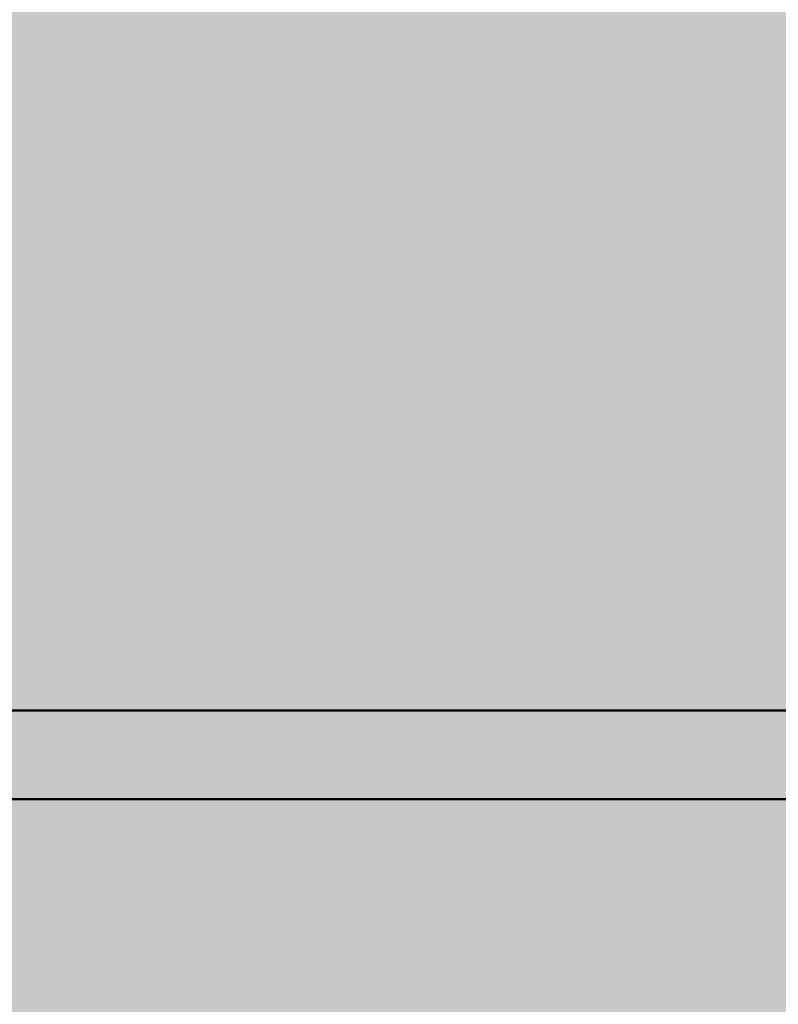
# Model space of a CAD drawing. Units: millimetres. Extents: x 0 to 2267, y 0 to 1823.
# Tile 134 of 256: x 1632 to 1675, y 1216 to 1271. Entities that reach past the tile are written whole.
import ezdxf

# ---------------------------------------------------------------- set-up
doc = ezdxf.new("R2010")
doc.units = ezdxf.units.MM
doc.header["$MEASUREMENT"] = 0
doc.layers.add('M-HATC', color=252, linetype='Continuous', lineweight=18)
doc.layers.add('M-OUTL', color=7, linetype='Continuous', lineweight=50)

msp = doc.modelspace()

# ---------------------------------------------------------------- hatches: boundary and pattern name
at = {"layer": 'M-HATC'}
h = msp.add_hatch(color=256, dxfattribs=at)
h.dxf.hatch_style = 1
h.paths.add_polyline_path([(2065.771, 1618.062, 0.236068), (2055.771, 1638.062), (1381.087, 1638.062, 0.236068), (1371.087, 1618.062), (1371.087, 1603.062), (2055.771, 1603.062), (2065.771, 1603.062)])
h.paths.add_polyline_path([(2062.772, 1550.296), (2062.772, 1560.296), (1374.086, 1560.296), (1374.086, 1550.296), (1374.086, 1540.296), (1384.086, 1540.296), (1389.086, 1540.296), (2062.772, 1540.296)])
h.paths.add_polyline_path([(1930.929, 1282.766), (1505.929, 1282.766), (1587.628, 1235.597, 0.131652), (1600.128, 1232.247), (1836.73, 1232.247, 0.131652), (1849.23, 1235.597)])
h.paths.add_polyline_path([(1930.929, 1117.417), (1905.929, 1117.417), (1505.929, 1117.417), (1505.929, 1077.417), (1930.929, 1077.417)])
h = msp.add_hatch(color=256, dxfattribs=at)
h.dxf.hatch_style = 1
h.paths.add_polyline_path([(2055.771, 1603.062), (1381.087, 1603.062), (1381.087, 1598.062), (2055.771, 1598.062)])
h.paths.add_polyline_path([(2055.771, 1598.062), (1381.087, 1598.062), (1381.087, 1593.062), (2055.771, 1593.062)])
h.paths.add_polyline_path([(2051.307, 1536.761), (1385.55, 1536.761), (1385.55, 1526.761), (1387.55, 1526.761), (1388.537, 1525.053), (1385.332, 1521.233), (1385.332, 1521.223), (2050.254, 1522.749), (2048.321, 1525.053), (2049.307, 1526.761), (2051.307, 1526.761)])
edge = h.paths.add_edge_path()
edge.add_arc((1847.535, 1379.149), 135, 222.60306, 222.89085, ccw=False)
edge.add_line((1748.166, 1287.766), (1683.092, 1287.766))
edge.add_arc((1583.724, 1379.149), 135, 317.10915, 317.39694, ccw=False)
edge.add_arc((1678.969, 1290.671), 5, 222.8909, 317.1091, ccw=False)
edge.add_arc((1774.213, 1379.149), 135, 222.60306, 222.89085, ccw=False)
edge.add_line((1674.845, 1287.766), (1609.771, 1287.766))
edge.add_arc((1510.403, 1379.149), 135, 317.10915, 317.39694, ccw=False)
edge.add_arc((1605.647, 1290.671), 5, 222.8909, 317.1091, ccw=False)
edge.add_arc((1700.892, 1379.149), 135, 222.60306, 222.89085, ccw=False)
edge.add_line((1601.524, 1287.766), (1536.45, 1287.766))
edge.add_arc((1437.081, 1379.149), 135, 317.10915, 317.39694, ccw=False)
edge.add_arc((1532.326, 1290.671), 5, 222.8909, 317.1091, ccw=False)
edge.add_arc((1627.571, 1379.149), 135, 222.60306, 222.89085, ccw=False)
edge.add_line((1528.203, 1287.766), (1505.929, 1287.766))
edge.add_spline(control_points=[(1505.929, 1287.766), (1504.262, 1287.766), (1504.262, 1282.766), (1505.929, 1282.766)], knot_values=[0, 0, 0, 0, 5, 5, 5, 5], degree=3, periodic=0)
edge.add_line((1505.929, 1282.766), (1930.929, 1282.766))
edge.add_spline(control_points=[(1930.929, 1282.766), (1932.596, 1282.766), (1932.596, 1287.766), (1930.929, 1287.766)], knot_values=[0, 0, 0, 0, 5, 5, 5, 5], degree=3, periodic=0)
edge.add_line((1930.929, 1287.766), (1903.056, 1287.766))
edge.add_arc((1803.688, 1379.149), 135, 317.10915, 317.39694, ccw=False)
edge.add_arc((1898.932, 1290.671), 5, 222.8909, 317.1091, ccw=False)
edge.add_arc((1994.177, 1379.149), 135, 222.60306, 222.89085, ccw=False)
edge.add_line((1894.809, 1287.766), (1829.735, 1287.766))
edge.add_arc((1730.366, 1379.149), 135, 317.10915, 317.39694, ccw=False)
edge.add_arc((1825.611, 1290.671), 5, 222.8909, 317.1091, ccw=False)
edge.add_arc((1920.856, 1379.149), 135, 222.60306, 222.89085, ccw=False)
edge.add_line((1821.487, 1287.766), (1756.413, 1287.766))
edge.add_arc((1657.045, 1379.149), 135, 317.10915, 317.39694, ccw=False)
edge.add_arc((1752.29, 1290.671), 5, 222.8909, 317.1091, ccw=False)
edge = h.paths.add_edge_path()
edge.add_spline(control_points=[(1843.429, 1227.247), (1845.096, 1227.247), (1845.096, 1232.247), (1843.429, 1232.247)], knot_values=[0, 0, 0, 0, 5, 5, 5, 5], degree=3, periodic=0)
edge.add_line((1843.429, 1232.247), (1593.429, 1232.247))
edge.add_spline(control_points=[(1593.429, 1232.247), (1591.762, 1232.247), (1591.762, 1227.247), (1593.429, 1227.247)], knot_values=[0, 0, 0, 0, 5, 5, 5, 5], degree=3, periodic=0)
edge.add_line((1593.429, 1227.247), (1843.429, 1227.247))
h.paths.add_polyline_path([(1905.929, 1127.417), (1530.929, 1127.417, 0.414214), (1520.929, 1117.417), (1530.929, 1117.417), (1915.929, 1117.417, 0.414214)])
edge = h.paths.add_edge_path()
edge.add_arc((1397.086, 1498.408), 12.73, 90.7821, 190.8787, ccw=False)
edge.add_line((1396.912, 1511.136), (1428.01, 1511.349))
edge.add_line((1428.01, 1511.349), (1433.01, 1511.349))
edge.add_line((1433.01, 1511.349), (1434.439, 1511.349))
edge.add_arc((1419.474, 1498.08), 20, 41.561, 74.0821)
edge.add_line((1424.959, 1517.314), (1399.935, 1517.256))
edge.add_spline(control_points=[(1399.931, 1517.256), (1399.884, 1517.213), (1399.833, 1517.169), (1399.777, 1517.124)], knot_values=[11.567499, 11.567499, 11.567499, 11.567499, 11.814249, 11.814249, 11.814249, 11.814249], degree=3, periodic=0)
edge.add_spline(control_points=[(1399.633, 1517.01), (1399.583, 1516.972), (1399.531, 1516.934), (1399.476, 1516.895)], knot_values=[11.167718, 11.167718, 11.167718, 11.167718, 11.365188, 11.365188, 11.365188, 11.365188], degree=3, periodic=0)
edge.add_spline(control_points=[(1399.34, 1516.8), (1399.151, 1516.672), (1398.938, 1516.538), (1398.704, 1516.399)], knot_values=[10.376405, 10.376405, 10.376405, 10.376405, 11.00994, 11.00994, 11.00994, 11.00994], degree=3, periodic=0)
edge.add_spline(control_points=[(1398.657, 1516.372), (1398.579, 1516.326), (1398.498, 1516.28), (1398.415, 1516.233)], knot_values=[10.125175, 10.125175, 10.125175, 10.125175, 10.334406, 10.334406, 10.334406, 10.334406], degree=3, periodic=0)
edge.add_spline(control_points=[(1398.264, 1516.149), (1398.196, 1516.111), (1398.126, 1516.073), (1398.055, 1516.035)], knot_values=[9.832246, 9.832246, 9.832246, 9.832246, 9.999658, 9.999658, 9.999658, 9.999658], degree=3, periodic=0)
edge.add_spline(control_points=[(1397.999, 1516.005), (1397.731, 1515.862), (1397.446, 1515.717), (1397.147, 1515.571)], knot_values=[9.161808, 9.161808, 9.161808, 9.161808, 9.787769, 9.787769, 9.787769, 9.787769], degree=3, periodic=0)
edge.add_spline(control_points=[(1397.147, 1515.571), (1396.842, 1515.423), (1396.522, 1515.274), (1396.191, 1515.126)], knot_values=[8.524455, 8.524455, 8.524455, 8.524455, 9.161808, 9.161808, 9.161808, 9.161808], degree=3, periodic=0)
edge.add_spline(control_points=[(1396.078, 1515.076), (1395.985, 1515.035), (1395.892, 1514.994), (1395.798, 1514.953)], knot_values=[8.275193, 8.275193, 8.275193, 8.275193, 8.451726, 8.451726, 8.451726, 8.451726], degree=3, periodic=0)
edge.add_spline(control_points=[(1395.602, 1514.869), (1395.5, 1514.826), (1395.397, 1514.782), (1395.293, 1514.739)], knot_values=[7.962917, 7.962917, 7.962917, 7.962917, 8.152764, 8.152764, 8.152764, 8.152764], degree=3, periodic=0)
edge.add_spline(control_points=[(1395.212, 1514.706), (1394.828, 1514.547), (1394.435, 1514.393), (1394.036, 1514.244)], knot_values=[7.21254, 7.21254, 7.21254, 7.21254, 7.913148, 7.913148, 7.913148, 7.913148], degree=3, periodic=0)
edge.add_spline(control_points=[(1394.036, 1514.244), (1393.708, 1514.121), (1393.375, 1514.003), (1393.043, 1513.889)], knot_values=[6.633733, 6.633733, 6.633733, 6.633733, 7.21254, 7.21254, 7.21254, 7.21254], degree=3, periodic=0)
edge.add_spline(control_points=[(1392.821, 1513.815), (1392.72, 1513.781), (1392.618, 1513.748), (1392.517, 1513.715)], knot_values=[6.328796, 6.328796, 6.328796, 6.328796, 6.505493, 6.505493, 6.505493, 6.505493], degree=3, periodic=0)
edge.add_spline(control_points=[(1392.517, 1513.715), (1392.319, 1513.652), (1392.121, 1513.59), (1391.924, 1513.531)], knot_values=[5.984605, 5.984605, 5.984605, 5.984605, 6.328796, 6.328796, 6.328796, 6.328796], degree=3, periodic=0)
edge.add_spline(control_points=[(1391.792, 1513.491), (1391.312, 1513.35), (1390.838, 1513.224), (1390.378, 1513.117)], knot_values=[5.066697, 5.066697, 5.066697, 5.066697, 5.907055, 5.907055, 5.907055, 5.907055], degree=3, periodic=0)
edge.add_spline(control_points=[(1390.378, 1513.117), (1390.18, 1513.071), (1389.984, 1513.028), (1389.791, 1512.99)], knot_values=[4.70367, 4.70367, 4.70367, 4.70367, 5.066695, 5.066695, 5.066695, 5.066695], degree=3, periodic=0)
edge.add_spline(control_points=[(1389.422, 1512.92), (1389.246, 1512.889), (1389.073, 1512.862), (1388.904, 1512.838)], knot_values=[4.130571, 4.130571, 4.130571, 4.130571, 4.469816, 4.469816, 4.469816, 4.469816], degree=3, periodic=0)
edge.add_spline(control_points=[(1388.904, 1512.838), (1388.591, 1512.795), (1388.291, 1512.764), (1388.007, 1512.749)], knot_values=[3.504031, 3.504031, 3.504031, 3.504031, 4.130571, 4.130571, 4.130571, 4.130571], degree=3, periodic=0)
edge.add_spline(control_points=[(1387.936, 1512.746), (1387.854, 1512.742), (1387.773, 1512.74), (1387.694, 1512.739)], knot_values=[3.268866, 3.268866, 3.268866, 3.268866, 3.451164, 3.451164, 3.451164, 3.451164], degree=3, periodic=0)
edge.add_spline(control_points=[(1387.335, 1512.744), (1387.208, 1512.75), (1387.085, 1512.76), (1386.967, 1512.774)], knot_values=[2.670686, 2.670686, 2.670686, 2.670686, 2.984, 2.984, 2.984, 2.984], degree=3, periodic=0)
edge.add_spline(control_points=[(1386.833, 1512.792), (1386.821, 1512.794), (1386.809, 1512.796), (1386.797, 1512.798)], knot_values=[2.516981, 2.516981, 2.516981, 2.516981, 2.549528, 2.549528, 2.549528, 2.549528], degree=3, periodic=0)
edge.add_spline(control_points=[(1386.453, 1512.873), (1386.426, 1512.881), (1386.399, 1512.889), (1386.373, 1512.897)], knot_values=[2.095869, 2.095869, 2.095869, 2.095869, 2.17941, 2.17941, 2.17941, 2.17941], degree=3, periodic=0)
edge.add_spline(control_points=[(1386.069, 1513.019), (1386.063, 1513.022), (1386.058, 1513.025), (1386.052, 1513.028)], knot_values=[1.72453, 1.72453, 1.72453, 1.72453, 1.745933, 1.745933, 1.745933, 1.745933], degree=3, periodic=0)
edge.add_arc((1399.474, 1498.08), 20, 131.8243, 180)
edge.add_arc((1630.334, 1505.548), 250.971, 181.70518, 236.42798)
edge.add_arc((1605.34, 1483.304), 218.782, 238.66083, 243.34961)
edge.add_arc((1647.091, 1510.359), 262.899, 183.12984, 237.85344, ccw=False)
h.paths.add_polyline_path([(1406.537, 1391.964, 0.149382), (1491.551, 1296.442, -0.129517)], flags=17)
edge = h.paths.add_edge_path()
edge.add_arc((2037.384, 1498.08), 20, 0, 48.2659)
edge.add_spline(control_points=[(2050.697, 1513.005), (2050.651, 1512.985), (2050.603, 1512.966), (2050.554, 1512.948)], knot_values=[1.835652, 1.835652, 1.835652, 1.835652, 2.000781, 2.000781, 2.000781, 2.000781], degree=3, periodic=0)
edge.add_spline(control_points=[(2050.462, 1512.917), (2050.479, 1512.922), (2050.496, 1512.928), (2050.513, 1512.934)], knot_values=[2.045477, 2.045477, 2.045477, 2.045477, 2.101389, 2.101389, 2.101389, 2.101389], degree=3, periodic=0)
edge.add_spline(control_points=[(2050.129, 1512.834), (2050.198, 1512.847), (2050.266, 1512.862), (2050.331, 1512.879)], knot_values=[2.237629, 2.237629, 2.237629, 2.237629, 2.435841, 2.435841, 2.435841, 2.435841], degree=3, periodic=0)
edge.add_spline(control_points=[(2050.095, 1512.828), (2050.106, 1512.83), (2050.118, 1512.832), (2050.129, 1512.834)], knot_values=[2.435841, 2.435841, 2.435841, 2.435841, 2.468321, 2.468321, 2.468321, 2.468321], degree=3, periodic=0)
edge.add_spline(control_points=[(2049.784, 1512.785), (2049.855, 1512.792), (2049.924, 1512.801), (2049.992, 1512.811)], knot_values=[2.563852, 2.563852, 2.563852, 2.563852, 2.748541, 2.748541, 2.748541, 2.748541], degree=3, periodic=0)
edge.add_spline(control_points=[(2049.405, 1512.762), (2049.536, 1512.765), (2049.663, 1512.773), (2049.784, 1512.785)], knot_values=[2.748541, 2.748541, 2.748541, 2.748541, 3.064882, 3.064882, 3.064882, 3.064882], degree=3, periodic=0)
edge.add_spline(control_points=[(2049.17, 1512.76), (2049.234, 1512.759), (2049.297, 1512.759), (2049.358, 1512.761)], knot_values=[3.102309, 3.102309, 3.102309, 3.102309, 3.2503, 3.2503, 3.2503, 3.2503], degree=3, periodic=0)
edge.add_spline(control_points=[(2048.857, 1512.769), (2048.964, 1512.764), (2049.068, 1512.761), (2049.17, 1512.76)], knot_values=[3.2503, 3.2503, 3.2503, 3.2503, 3.486069, 3.486069, 3.486069, 3.486069], degree=3, periodic=0)
edge.add_spline(control_points=[(2048.692, 1512.779), (2048.373, 1512.801), (2048.035, 1512.841), (2047.682, 1512.897)], knot_values=[3.606429, 3.606429, 3.606429, 3.606429, 4.2989, 4.2989, 4.2989, 4.2989], degree=3, periodic=0)
edge.add_spline(control_points=[(2047.682, 1512.897), (2047.546, 1512.919), (2047.408, 1512.942), (2047.268, 1512.969)], knot_values=[4.2989, 4.2989, 4.2989, 4.2989, 4.565769, 4.565769, 4.565769, 4.565769], degree=3, periodic=0)
edge.add_spline(control_points=[(2047.268, 1512.969), (2047.145, 1512.991), (2047.021, 1513.016), (2046.895, 1513.042)], knot_values=[4.565769, 4.565769, 4.565769, 4.565769, 4.799971, 4.799971, 4.799971, 4.799971], degree=3, periodic=0)
edge.add_spline(control_points=[(2046.895, 1513.042), (2046.529, 1513.119), (2046.151, 1513.209), (2045.768, 1513.311)], knot_values=[4.799971, 4.799971, 4.799971, 4.799971, 5.483718, 5.483718, 5.483718, 5.483718], degree=3, periodic=0)
edge.add_spline(control_points=[(2045.768, 1513.311), (2045.372, 1513.415), (2044.97, 1513.532), (2044.566, 1513.659)], knot_values=[5.483718, 5.483718, 5.483718, 5.483718, 6.187866, 6.187866, 6.187866, 6.187866], degree=3, periodic=0)
edge.add_spline(control_points=[(2044.566, 1513.659), (2044.415, 1513.706), (2044.263, 1513.755), (2044.112, 1513.805)], knot_values=[6.187866, 6.187866, 6.187866, 6.187866, 6.451551, 6.451551, 6.451551, 6.451551], degree=3, periodic=0)
edge.add_spline(control_points=[(2044.112, 1513.805), (2043.997, 1513.843), (2043.882, 1513.881), (2043.767, 1513.92)], knot_values=[6.451551, 6.451551, 6.451551, 6.451551, 6.651434, 6.651434, 6.651434, 6.651434], degree=3, periodic=0)
edge.add_spline(control_points=[(2043.767, 1513.92), (2043.372, 1514.055), (2042.977, 1514.198), (2042.589, 1514.346)], knot_values=[6.651434, 6.651434, 6.651434, 6.651434, 7.338879, 7.338879, 7.338879, 7.338879], degree=3, periodic=0)
edge.add_spline(control_points=[(2042.589, 1514.346), (2042.164, 1514.507), (2041.746, 1514.675), (2041.341, 1514.846)], knot_values=[7.338879, 7.338879, 7.338879, 7.338879, 8.089209, 8.089209, 8.089209, 8.089209], degree=3, periodic=0)
edge.add_spline(control_points=[(2041.341, 1514.846), (2041.103, 1514.946), (2040.869, 1515.048), (2040.64, 1515.15)], knot_values=[8.089209, 8.089209, 8.089209, 8.089209, 8.529587, 8.529587, 8.529587, 8.529587], degree=3, periodic=0)
edge.add_spline(control_points=[(2040.51, 1515.209), (2040.082, 1515.402), (2039.675, 1515.597), (2039.295, 1515.789)], knot_values=[8.613818, 8.613818, 8.613818, 8.613818, 9.44571, 9.44571, 9.44571, 9.44571], degree=3, periodic=0)
edge.add_spline(control_points=[(2039.295, 1515.789), (2039.062, 1515.907), (2038.839, 1516.025), (2038.629, 1516.14)], knot_values=[9.44571, 9.44571, 9.44571, 9.44571, 9.956404, 9.956404, 9.956404, 9.956404], degree=3, periodic=0)
edge.add_spline(control_points=[(2038.629, 1516.14), (2038.519, 1516.2), (2038.412, 1516.26), (2038.309, 1516.319)], knot_values=[9.956404, 9.956404, 9.956404, 9.956404, 10.223542, 10.223542, 10.223542, 10.223542], degree=3, periodic=0)
edge.add_spline(control_points=[(2038.309, 1516.319), (2038.214, 1516.374), (2038.122, 1516.428), (2038.033, 1516.481)], knot_values=[10.223542, 10.223542, 10.223542, 10.223542, 10.47051, 10.47051, 10.47051, 10.47051], degree=3, periodic=0)
edge.add_spline(control_points=[(2038.033, 1516.481), (2037.786, 1516.63), (2037.564, 1516.773), (2037.372, 1516.909)], knot_values=[10.47051, 10.47051, 10.47051, 10.47051, 11.15767, 11.15767, 11.15767, 11.15767], degree=3, periodic=0)
edge.add_spline(control_points=[(2037.372, 1516.909), (2037.279, 1516.975), (2037.193, 1517.04), (2037.114, 1517.102)], knot_values=[11.15767, 11.15767, 11.15767, 11.15767, 11.49227, 11.49227, 11.49227, 11.49227], degree=3, periodic=0)
edge.add_spline(control_points=[(2036.856, 1517.326), (2036.915, 1517.269), (2036.981, 1517.21), (2037.056, 1517.149)], knot_values=[11.577341, 11.577341, 11.577341, 11.577341, 11.91035, 11.91035, 11.91035, 11.91035], degree=3, periodic=0)
edge.add_spline(control_points=[(2036.807, 1517.375), (2036.823, 1517.359), (2036.839, 1517.342), (2036.856, 1517.326)], knot_values=[11.91035, 11.91035, 11.91035, 11.91035, 12.007402, 12.007402, 12.007402, 12.007402], degree=3, periodic=0)
edge.add_spline(control_points=[(2036.702, 1517.494), (2036.71, 1517.483), (2036.72, 1517.472), (2036.729, 1517.461)], knot_values=[12.184155, 12.184155, 12.184155, 12.184155, 12.255409, 12.255409, 12.255409, 12.255409], degree=3, periodic=0)
edge.add_spline(control_points=[(2036.616, 1517.621), (2036.62, 1517.613), (2036.624, 1517.606), (2036.629, 1517.598)], knot_values=[12.487913, 12.487913, 12.487913, 12.487913, 12.541035, 12.541035, 12.541035, 12.541035], degree=3, periodic=0)
edge.add_spline(control_points=[(2036.563, 1517.786), (2036.564, 1517.779), (2036.564, 1517.773), (2036.565, 1517.766)], knot_values=[12.911761, 12.911761, 12.911761, 12.911761, 12.968286, 12.968286, 12.968286, 12.968286], degree=3, periodic=0)
edge.add_spline(control_points=[(2036.617, 1517.93), (2036.612, 1517.926), (2036.609, 1517.921), (2036.605, 1517.916)], knot_values=[13.382527, 13.382527, 13.382527, 13.382527, 13.433791, 13.433791, 13.433791, 13.433791], degree=3, periodic=0)
edge.add_spline(control_points=[(2036.749, 1518.017), (2036.736, 1518.012), (2036.724, 1518.006), (2036.712, 1518)], knot_values=[13.726299, 13.726299, 13.726299, 13.726299, 13.809928, 13.809928, 13.809928, 13.809928], degree=3, periodic=0)
edge.add_spline(control_points=[(2036.86, 1518.053), (2036.839, 1518.047), (2036.818, 1518.042), (2036.799, 1518.035)], knot_values=[13.910887, 13.910887, 13.910887, 13.910887, 14.02153, 14.02153, 14.02153, 14.02153], degree=3, periodic=0)
edge.add_line((2036.964, 1518.08), (2032.384, 1518.08))
edge.add_line((2032.384, 1518.08), (2027.384, 1518.08))
edge.add_line((2027.384, 1518.08), (2022.384, 1518.08))
edge.add_line((2022.384, 1518.08), (2017.384, 1518.08))
edge.add_arc((2017.384, 1498.08), 20, 90, 138.439)
edge.add_line((2002.419, 1511.349), (2003.848, 1511.349))
edge.add_line((2003.848, 1511.349), (2008.848, 1511.349))
edge.add_line((2008.848, 1511.349), (2039.772, 1511.138))
edge.add_arc((2039.772, 1498.408), 12.73, -10.8787, 90, ccw=False)
edge.add_arc((1789.767, 1510.359), 262.899, 302.14656, 356.87016, ccw=False)
edge.add_arc((1831.518, 1483.304), 218.782, 296.65039, 301.33917)
edge.add_arc((1806.524, 1505.548), 250.971, 303.57202, 358.29482)
h.paths.add_polyline_path([(2030.321, 1391.964, -0.129517), (1945.307, 1296.442, 0.149382)], flags=17)
edge = h.paths.add_edge_path()
edge.add_spline(control_points=[(2037.246, 1518.082), (2037.29, 1518.081), (2037.336, 1518.08), (2037.384, 1518.08)], knot_values=[0.000012, 0.000012, 0.000012, 0.000012, 0.144754, 0.144754, 0.144754, 0.144754], degree=3, periodic=0)
edge.add_line((2037.336, 1518.08), (2037.01, 1518.08))
edge.add_spline(control_points=[(2037.01, 1518.08), (2036.982, 1518.077), (2036.956, 1518.073), (2036.931, 1518.068)], knot_values=[14.13465, 14.13465, 14.13465, 14.13465, 14.247197, 14.247197, 14.247197, 14.247197], degree=3, periodic=0)
edge.add_spline(control_points=[(2036.931, 1518.068), (2036.928, 1518.067), (2036.924, 1518.067), (2036.921, 1518.066)], knot_values=[14.118315, 14.118315, 14.118315, 14.118315, 14.13465, 14.13465, 14.13465, 14.13465], degree=3, periodic=0)
edge.add_spline(control_points=[(2036.921, 1518.066), (2036.912, 1518.064), (2036.903, 1518.063), (2036.895, 1518.061)], knot_values=[14.078086, 14.078086, 14.078086, 14.078086, 14.118315, 14.118315, 14.118315, 14.118315], degree=3, periodic=0)
edge.add_spline(control_points=[(2036.895, 1518.061), (2036.883, 1518.058), (2036.872, 1518.056), (2036.86, 1518.053)], knot_values=[14.02153, 14.02153, 14.02153, 14.02153, 14.078086, 14.078086, 14.078086, 14.078086], degree=3, periodic=0)
edge.add_spline(control_points=[(2036.86, 1518.053), (2036.839, 1518.047), (2036.818, 1518.042), (2036.799, 1518.035)], knot_values=[13.910887, 13.910887, 13.910887, 13.910887, 14.02153, 14.02153, 14.02153, 14.02153], degree=3, periodic=0)
edge.add_spline(control_points=[(2036.799, 1518.035), (2036.798, 1518.035), (2036.797, 1518.035), (2036.797, 1518.035)], knot_values=[13.906906, 13.906906, 13.906906, 13.906906, 13.910887, 13.910887, 13.910887, 13.910887], degree=3, periodic=0)
edge.add_spline(control_points=[(2036.797, 1518.035), (2036.788, 1518.032), (2036.78, 1518.029), (2036.772, 1518.026)], knot_values=[13.857826, 13.857826, 13.857826, 13.857826, 13.906906, 13.906906, 13.906906, 13.906906], degree=3, periodic=0)
edge.add_spline(control_points=[(2036.772, 1518.026), (2036.764, 1518.023), (2036.756, 1518.02), (2036.749, 1518.017)], knot_values=[13.809928, 13.809928, 13.809928, 13.809928, 13.857826, 13.857826, 13.857826, 13.857826], degree=3, periodic=0)
edge.add_spline(control_points=[(2036.749, 1518.017), (2036.736, 1518.012), (2036.724, 1518.006), (2036.712, 1518)], knot_values=[13.726299, 13.726299, 13.726299, 13.726299, 13.809928, 13.809928, 13.809928, 13.809928], degree=3, periodic=0)
edge.add_spline(control_points=[(2036.712, 1518), (2036.712, 1518), (2036.712, 1518), (2036.711, 1518)], knot_values=[13.723993, 13.723993, 13.723993, 13.723993, 13.726299, 13.726299, 13.726299, 13.726299], degree=3, periodic=0)
edge.add_spline(control_points=[(2036.711, 1518), (2036.706, 1517.997), (2036.701, 1517.994), (2036.696, 1517.992)], knot_values=[13.686536, 13.686536, 13.686536, 13.686536, 13.723993, 13.723993, 13.723993, 13.723993], degree=3, periodic=0)
edge.add_spline(control_points=[(2036.696, 1517.992), (2036.692, 1517.989), (2036.687, 1517.987), (2036.683, 1517.984)], knot_values=[13.651251, 13.651251, 13.651251, 13.651251, 13.686536, 13.686536, 13.686536, 13.686536], degree=3, periodic=0)
edge.add_spline(control_points=[(2036.683, 1517.984), (2036.676, 1517.98), (2036.67, 1517.976), (2036.664, 1517.971)], knot_values=[13.596804, 13.596804, 13.596804, 13.596804, 13.651251, 13.651251, 13.651251, 13.651251], degree=3, periodic=0)
edge.add_spline(control_points=[(2036.664, 1517.971), (2036.664, 1517.971), (2036.663, 1517.971), (2036.663, 1517.971)], knot_values=[13.593956, 13.593956, 13.593956, 13.593956, 13.596804, 13.596804, 13.596804, 13.596804], degree=3, periodic=0)
edge.add_spline(control_points=[(2036.663, 1517.971), (2036.66, 1517.969), (2036.658, 1517.967), (2036.655, 1517.965)], knot_values=[13.570322, 13.570322, 13.570322, 13.570322, 13.593956, 13.593956, 13.593956, 13.593956], degree=3, periodic=0)
edge.add_spline(control_points=[(2036.655, 1517.965), (2036.653, 1517.963), (2036.65, 1517.961), (2036.647, 1517.959)], knot_values=[13.545477, 13.545477, 13.545477, 13.545477, 13.570322, 13.570322, 13.570322, 13.570322], degree=3, periodic=0)
edge.add_spline(control_points=[(2036.647, 1517.959), (2036.647, 1517.959), (2036.647, 1517.959), (2036.647, 1517.959)], knot_values=[13.543931, 13.543931, 13.543931, 13.543931, 13.545477, 13.545477, 13.545477, 13.545477], degree=3, periodic=0)
edge.add_spline(control_points=[(2036.647, 1517.959), (2036.641, 1517.954), (2036.636, 1517.949), (2036.631, 1517.945)], knot_values=[13.488237, 13.488237, 13.488237, 13.488237, 13.543931, 13.543931, 13.543931, 13.543931], degree=3, periodic=0)
edge.add_spline(control_points=[(2036.631, 1517.945), (2036.628, 1517.942), (2036.626, 1517.94), (2036.623, 1517.937)], knot_values=[13.460307, 13.460307, 13.460307, 13.460307, 13.488237, 13.488237, 13.488237, 13.488237], degree=3, periodic=0)
edge.add_spline(control_points=[(2036.623, 1517.937), (2036.622, 1517.936), (2036.62, 1517.934), (2036.618, 1517.932)], knot_values=[13.439712, 13.439712, 13.439712, 13.439712, 13.460307, 13.460307, 13.460307, 13.460307], degree=3, periodic=0)
edge.add_spline(control_points=[(2036.618, 1517.932), (2036.618, 1517.931), (2036.617, 1517.931), (2036.617, 1517.93)], knot_values=[13.433791, 13.433791, 13.433791, 13.433791, 13.439712, 13.439712, 13.439712, 13.439712], degree=3, periodic=0)
edge.add_spline(control_points=[(2036.617, 1517.93), (2036.612, 1517.926), (2036.609, 1517.921), (2036.605, 1517.916)], knot_values=[13.382527, 13.382527, 13.382527, 13.382527, 13.433791, 13.433791, 13.433791, 13.433791], degree=3, periodic=0)
edge.add_spline(control_points=[(2036.605, 1517.916), (2036.603, 1517.913), (2036.6, 1517.91), (2036.598, 1517.907)], knot_values=[13.350017, 13.350017, 13.350017, 13.350017, 13.382527, 13.382527, 13.382527, 13.382527], degree=3, periodic=0)
edge.add_spline(control_points=[(2036.598, 1517.907), (2036.597, 1517.906), (2036.596, 1517.904), (2036.595, 1517.903)], knot_values=[13.333922, 13.333922, 13.333922, 13.333922, 13.350017, 13.350017, 13.350017, 13.350017], degree=3, periodic=0)
edge.add_spline(control_points=[(2036.595, 1517.903), (2036.595, 1517.902), (2036.594, 1517.901), (2036.593, 1517.9)], knot_values=[13.323828, 13.323828, 13.323828, 13.323828, 13.333922, 13.333922, 13.333922, 13.333922], degree=3, periodic=0)
edge.add_spline(control_points=[(2036.593, 1517.9), (2036.59, 1517.895), (2036.588, 1517.891), (2036.585, 1517.886)], knot_values=[13.277545, 13.277545, 13.277545, 13.277545, 13.323828, 13.323828, 13.323828, 13.323828], degree=3, periodic=0)
edge.add_spline(control_points=[(2036.585, 1517.886), (2036.584, 1517.883), (2036.582, 1517.879), (2036.58, 1517.875)], knot_values=[13.240119, 13.240119, 13.240119, 13.240119, 13.277545, 13.277545, 13.277545, 13.277545], degree=3, periodic=0)
edge.add_spline(control_points=[(2036.58, 1517.875), (2036.58, 1517.874), (2036.579, 1517.873), (2036.578, 1517.872)], knot_values=[13.228211, 13.228211, 13.228211, 13.228211, 13.240119, 13.240119, 13.240119, 13.240119], degree=3, periodic=0)
edge.add_spline(control_points=[(2036.578, 1517.872), (2036.578, 1517.87), (2036.577, 1517.869), (2036.577, 1517.868)], knot_values=[13.215717, 13.215717, 13.215717, 13.215717, 13.228211, 13.228211, 13.228211, 13.228211], degree=3, periodic=0)
edge.add_spline(control_points=[(2036.577, 1517.868), (2036.575, 1517.864), (2036.574, 1517.86), (2036.573, 1517.857)], knot_values=[13.179847, 13.179847, 13.179847, 13.179847, 13.215717, 13.215717, 13.215717, 13.215717], degree=3, periodic=0)
edge.add_spline(control_points=[(2036.573, 1517.857), (2036.571, 1517.851), (2036.57, 1517.846), (2036.569, 1517.841)], knot_values=[13.132017, 13.132017, 13.132017, 13.132017, 13.179847, 13.179847, 13.179847, 13.179847], degree=3, periodic=0)
edge.add_spline(control_points=[(2036.569, 1517.841), (2036.568, 1517.84), (2036.568, 1517.839), (2036.568, 1517.838)], knot_values=[13.122482, 13.122482, 13.122482, 13.122482, 13.132017, 13.132017, 13.132017, 13.132017], degree=3, periodic=0)
edge.add_spline(control_points=[(2036.568, 1517.838), (2036.568, 1517.836), (2036.567, 1517.835), (2036.567, 1517.833)], knot_values=[13.105592, 13.105592, 13.105592, 13.105592, 13.122482, 13.122482, 13.122482, 13.122482], degree=3, periodic=0)
edge.add_spline(control_points=[(2036.567, 1517.833), (2036.566, 1517.829), (2036.566, 1517.826), (2036.565, 1517.822)], knot_values=[13.074063, 13.074063, 13.074063, 13.074063, 13.105592, 13.105592, 13.105592, 13.105592], degree=3, periodic=0)
edge.add_spline(control_points=[(2036.565, 1517.822), (2036.565, 1517.822), (2036.565, 1517.822), (2036.565, 1517.822)], knot_values=[13.074043, 13.074043, 13.074043, 13.074043, 13.074063, 13.074063, 13.074063, 13.074063], degree=3, periodic=0)
edge.add_spline(control_points=[(2036.565, 1517.822), (2036.564, 1517.816), (2036.564, 1517.811), (2036.564, 1517.805)], knot_values=[13.021884, 13.021884, 13.021884, 13.021884, 13.074043, 13.074043, 13.074043, 13.074043], degree=3, periodic=0)
edge.add_spline(control_points=[(2036.564, 1517.805), (2036.564, 1517.804), (2036.564, 1517.803), (2036.564, 1517.803)], knot_values=[13.01674, 13.01674, 13.01674, 13.01674, 13.021884, 13.021884, 13.021884, 13.021884], degree=3, periodic=0)
edge.add_spline(control_points=[(2036.564, 1517.803), (2036.563, 1517.801), (2036.563, 1517.798), (2036.563, 1517.796)], knot_values=[12.996438, 12.996438, 12.996438, 12.996438, 13.01674, 13.01674, 13.01674, 13.01674], degree=3, periodic=0)
edge.add_spline(control_points=[(2036.563, 1517.796), (2036.563, 1517.793), (2036.563, 1517.789), (2036.563, 1517.786)], knot_values=[12.968286, 12.968286, 12.968286, 12.968286, 12.996438, 12.996438, 12.996438, 12.996438], degree=3, periodic=0)
edge.add_spline(control_points=[(2036.563, 1517.786), (2036.564, 1517.779), (2036.564, 1517.773), (2036.565, 1517.766)], knot_values=[12.911761, 12.911761, 12.911761, 12.911761, 12.968286, 12.968286, 12.968286, 12.968286], degree=3, periodic=0)
edge.add_spline(control_points=[(2036.565, 1517.766), (2036.565, 1517.766), (2036.565, 1517.766), (2036.565, 1517.766)], knot_values=[12.911017, 12.911017, 12.911017, 12.911017, 12.911761, 12.911761, 12.911761, 12.911761], degree=3, periodic=0)
edge.add_spline(control_points=[(2036.565, 1517.766), (2036.565, 1517.762), (2036.566, 1517.759), (2036.566, 1517.756)], knot_values=[12.88528, 12.88528, 12.88528, 12.88528, 12.911017, 12.911017, 12.911017, 12.911017], degree=3, periodic=0)
edge.add_spline(control_points=[(2036.566, 1517.756), (2036.567, 1517.753), (2036.567, 1517.751), (2036.568, 1517.748)], knot_values=[12.862519, 12.862519, 12.862519, 12.862519, 12.88528, 12.88528, 12.88528, 12.88528], degree=3, periodic=0)
edge.add_spline(control_points=[(2036.568, 1517.748), (2036.568, 1517.747), (2036.568, 1517.747), (2036.568, 1517.746)], knot_values=[12.858885, 12.858885, 12.858885, 12.858885, 12.862519, 12.862519, 12.862519, 12.862519], degree=3, periodic=0)
edge.add_spline(control_points=[(2036.568, 1517.746), (2036.569, 1517.74), (2036.571, 1517.733), (2036.572, 1517.726)], knot_values=[12.8053, 12.8053, 12.8053, 12.8053, 12.858885, 12.858885, 12.858885, 12.858885], degree=3, periodic=0)
edge.add_spline(control_points=[(2036.572, 1517.726), (2036.573, 1517.723), (2036.574, 1517.719), (2036.576, 1517.715)], knot_values=[12.775176, 12.775176, 12.775176, 12.775176, 12.8053, 12.8053, 12.8053, 12.8053], degree=3, periodic=0)
edge.add_spline(control_points=[(2036.576, 1517.715), (2036.576, 1517.713), (2036.577, 1517.71), (2036.578, 1517.708)], knot_values=[12.756759, 12.756759, 12.756759, 12.756759, 12.775176, 12.775176, 12.775176, 12.775176], degree=3, periodic=0)
edge.add_spline(control_points=[(2036.578, 1517.708), (2036.578, 1517.707), (2036.578, 1517.706), (2036.579, 1517.705)], knot_values=[12.748742, 12.748742, 12.748742, 12.748742, 12.756759, 12.756759, 12.756759, 12.756759], degree=3, periodic=0)
edge.add_spline(control_points=[(2036.579, 1517.705), (2036.581, 1517.698), (2036.583, 1517.692), (2036.586, 1517.685)], knot_values=[12.69959, 12.69959, 12.69959, 12.69959, 12.748742, 12.748742, 12.748742, 12.748742], degree=3, periodic=0)
edge.add_spline(control_points=[(2036.586, 1517.685), (2036.588, 1517.68), (2036.59, 1517.675), (2036.592, 1517.669)], knot_values=[12.659038, 12.659038, 12.659038, 12.659038, 12.69959, 12.69959, 12.69959, 12.69959], degree=3, periodic=0)
edge.add_spline(control_points=[(2036.592, 1517.669), (2036.594, 1517.665), (2036.596, 1517.66), (2036.598, 1517.656)], knot_values=[12.626806, 12.626806, 12.626806, 12.626806, 12.659038, 12.659038, 12.659038, 12.659038], degree=3, periodic=0)
edge.add_spline(control_points=[(2036.598, 1517.656), (2036.598, 1517.655), (2036.599, 1517.654), (2036.599, 1517.653)], knot_values=[12.619394, 12.619394, 12.619394, 12.619394, 12.626806, 12.626806, 12.626806, 12.626806], degree=3, periodic=0)
edge.add_spline(control_points=[(2036.599, 1517.653), (2036.604, 1517.642), (2036.61, 1517.632), (2036.616, 1517.621)], knot_values=[12.541039, 12.541039, 12.541039, 12.541039, 12.619394, 12.619394, 12.619394, 12.619394], degree=3, periodic=0)
edge.add_spline(control_points=[(2036.616, 1517.621), (2036.616, 1517.621), (2036.616, 1517.621), (2036.616, 1517.621)], knot_values=[12.541035, 12.541035, 12.541035, 12.541035, 12.541039, 12.541039, 12.541039, 12.541039], degree=3, periodic=0)
edge.add_spline(control_points=[(2036.616, 1517.621), (2036.62, 1517.613), (2036.624, 1517.606), (2036.629, 1517.598)], knot_values=[12.487913, 12.487913, 12.487913, 12.487913, 12.541035, 12.541035, 12.541035, 12.541035], degree=3, periodic=0)
edge.add_spline(control_points=[(2036.629, 1517.598), (2036.633, 1517.592), (2036.637, 1517.585), (2036.641, 1517.579)], knot_values=[12.443982, 12.443982, 12.443982, 12.443982, 12.487913, 12.487913, 12.487913, 12.487913], degree=3, periodic=0)
edge.add_spline(control_points=[(2036.641, 1517.579), (2036.641, 1517.578), (2036.642, 1517.576), (2036.643, 1517.575)], knot_values=[12.434996, 12.434996, 12.434996, 12.434996, 12.443982, 12.443982, 12.443982, 12.443982], degree=3, periodic=0)
edge.add_spline(control_points=[(2036.643, 1517.575), (2036.653, 1517.56), (2036.664, 1517.544), (2036.676, 1517.528)], knot_values=[12.329647, 12.329647, 12.329647, 12.329647, 12.434996, 12.434996, 12.434996, 12.434996], degree=3, periodic=0)
edge.add_spline(control_points=[(2036.676, 1517.528), (2036.684, 1517.517), (2036.693, 1517.505), (2036.702, 1517.494)], knot_values=[12.255409, 12.255409, 12.255409, 12.255409, 12.329647, 12.329647, 12.329647, 12.329647], degree=3, periodic=0)
edge.add_spline(control_points=[(2036.702, 1517.494), (2036.71, 1517.483), (2036.72, 1517.472), (2036.729, 1517.461)], knot_values=[12.184155, 12.184155, 12.184155, 12.184155, 12.255409, 12.255409, 12.255409, 12.255409], degree=3, periodic=0)
edge.add_spline(control_points=[(2036.729, 1517.461), (2036.744, 1517.444), (2036.759, 1517.426), (2036.775, 1517.409)], knot_values=[12.075961, 12.075961, 12.075961, 12.075961, 12.184155, 12.184155, 12.184155, 12.184155], degree=3, periodic=0)
edge.add_spline(control_points=[(2036.775, 1517.409), (2036.776, 1517.407), (2036.777, 1517.406), (2036.778, 1517.405)], knot_values=[12.069502, 12.069502, 12.069502, 12.069502, 12.075961, 12.075961, 12.075961, 12.075961], degree=3, periodic=0)
edge.add_spline(control_points=[(2036.778, 1517.405), (2036.788, 1517.395), (2036.797, 1517.385), (2036.807, 1517.375)], knot_values=[12.007402, 12.007402, 12.007402, 12.007402, 12.069502, 12.069502, 12.069502, 12.069502], degree=3, periodic=0)
edge.add_spline(control_points=[(2036.807, 1517.375), (2036.823, 1517.359), (2036.839, 1517.342), (2036.856, 1517.326)], knot_values=[11.91035, 11.91035, 11.91035, 11.91035, 12.007402, 12.007402, 12.007402, 12.007402], degree=3, periodic=0)
edge.add_spline(control_points=[(2036.856, 1517.326), (2036.915, 1517.269), (2036.981, 1517.21), (2037.056, 1517.149)], knot_values=[11.577341, 11.577341, 11.577341, 11.577341, 11.91035, 11.91035, 11.91035, 11.91035], degree=3, periodic=0)
edge.add_spline(control_points=[(2037.056, 1517.149), (2037.075, 1517.134), (2037.094, 1517.118), (2037.114, 1517.102)], knot_values=[11.49227, 11.49227, 11.49227, 11.49227, 11.577341, 11.577341, 11.577341, 11.577341], degree=3, periodic=0)
edge.add_spline(control_points=[(2037.114, 1517.102), (2037.193, 1517.04), (2037.279, 1516.975), (2037.372, 1516.909)], knot_values=[11.15767, 11.15767, 11.15767, 11.15767, 11.49227, 11.49227, 11.49227, 11.49227], degree=3, periodic=0)
edge.add_spline(control_points=[(2037.372, 1516.909), (2037.564, 1516.773), (2037.786, 1516.63), (2038.033, 1516.481)], knot_values=[10.47051, 10.47051, 10.47051, 10.47051, 11.15767, 11.15767, 11.15767, 11.15767], degree=3, periodic=0)
edge.add_spline(control_points=[(2038.033, 1516.481), (2038.122, 1516.428), (2038.214, 1516.374), (2038.309, 1516.319)], knot_values=[10.223542, 10.223542, 10.223542, 10.223542, 10.47051, 10.47051, 10.47051, 10.47051], degree=3, periodic=0)
edge.add_spline(control_points=[(2038.309, 1516.319), (2038.412, 1516.26), (2038.519, 1516.2), (2038.629, 1516.14)], knot_values=[9.956404, 9.956404, 9.956404, 9.956404, 10.223542, 10.223542, 10.223542, 10.223542], degree=3, periodic=0)
edge.add_spline(control_points=[(2038.629, 1516.14), (2038.839, 1516.025), (2039.062, 1515.907), (2039.295, 1515.789)], knot_values=[9.44571, 9.44571, 9.44571, 9.44571, 9.956404, 9.956404, 9.956404, 9.956404], degree=3, periodic=0)
edge.add_spline(control_points=[(2039.295, 1515.789), (2039.675, 1515.597), (2040.082, 1515.402), (2040.51, 1515.209)], knot_values=[8.613818, 8.613818, 8.613818, 8.613818, 9.44571, 9.44571, 9.44571, 9.44571], degree=3, periodic=0)
edge.add_spline(control_points=[(2040.51, 1515.209), (2040.553, 1515.189), (2040.597, 1515.17), (2040.64, 1515.15)], knot_values=[8.529587, 8.529587, 8.529587, 8.529587, 8.613818, 8.613818, 8.613818, 8.613818], degree=3, periodic=0)
edge.add_spline(control_points=[(2040.64, 1515.15), (2040.869, 1515.048), (2041.103, 1514.946), (2041.341, 1514.846)], knot_values=[8.089209, 8.089209, 8.089209, 8.089209, 8.529587, 8.529587, 8.529587, 8.529587], degree=3, periodic=0)
edge.add_spline(control_points=[(2041.341, 1514.846), (2041.746, 1514.675), (2042.164, 1514.507), (2042.589, 1514.346)], knot_values=[7.338879, 7.338879, 7.338879, 7.338879, 8.089209, 8.089209, 8.089209, 8.089209], degree=3, periodic=0)
edge.add_spline(control_points=[(2042.589, 1514.346), (2042.977, 1514.198), (2043.372, 1514.055), (2043.767, 1513.92)], knot_values=[6.651434, 6.651434, 6.651434, 6.651434, 7.338879, 7.338879, 7.338879, 7.338879], degree=3, periodic=0)
edge.add_spline(control_points=[(2043.767, 1513.92), (2043.882, 1513.881), (2043.997, 1513.843), (2044.112, 1513.805)], knot_values=[6.451551, 6.451551, 6.451551, 6.451551, 6.651434, 6.651434, 6.651434, 6.651434], degree=3, periodic=0)
edge.add_spline(control_points=[(2044.112, 1513.805), (2044.263, 1513.755), (2044.415, 1513.706), (2044.566, 1513.659)], knot_values=[6.187866, 6.187866, 6.187866, 6.187866, 6.451551, 6.451551, 6.451551, 6.451551], degree=3, periodic=0)
edge.add_spline(control_points=[(2044.566, 1513.659), (2044.97, 1513.532), (2045.372, 1513.415), (2045.768, 1513.311)], knot_values=[5.483718, 5.483718, 5.483718, 5.483718, 6.187866, 6.187866, 6.187866, 6.187866], degree=3, periodic=0)
edge.add_spline(control_points=[(2045.768, 1513.311), (2046.151, 1513.209), (2046.529, 1513.119), (2046.895, 1513.042)], knot_values=[4.799971, 4.799971, 4.799971, 4.799971, 5.483718, 5.483718, 5.483718, 5.483718], degree=3, periodic=0)
edge.add_spline(control_points=[(2046.895, 1513.042), (2047.021, 1513.016), (2047.145, 1512.991), (2047.268, 1512.969)], knot_values=[4.565769, 4.565769, 4.565769, 4.565769, 4.799971, 4.799971, 4.799971, 4.799971], degree=3, periodic=0)
edge.add_spline(control_points=[(2047.268, 1512.969), (2047.408, 1512.942), (2047.546, 1512.919), (2047.682, 1512.897)], knot_values=[4.2989, 4.2989, 4.2989, 4.2989, 4.565769, 4.565769, 4.565769, 4.565769], degree=3, periodic=0)
edge.add_spline(control_points=[(2047.682, 1512.897), (2048.035, 1512.841), (2048.373, 1512.801), (2048.692, 1512.779)], knot_values=[3.606429, 3.606429, 3.606429, 3.606429, 4.2989, 4.2989, 4.2989, 4.2989], degree=3, periodic=0)
edge.add_spline(control_points=[(2048.692, 1512.779), (2048.748, 1512.775), (2048.803, 1512.772), (2048.857, 1512.769)], knot_values=[3.486069, 3.486069, 3.486069, 3.486069, 3.606429, 3.606429, 3.606429, 3.606429], degree=3, periodic=0)
edge.add_spline(control_points=[(2048.857, 1512.769), (2048.964, 1512.764), (2049.068, 1512.761), (2049.17, 1512.76)], knot_values=[3.2503, 3.2503, 3.2503, 3.2503, 3.486069, 3.486069, 3.486069, 3.486069], degree=3, periodic=0)
edge.add_spline(control_points=[(2049.17, 1512.76), (2049.234, 1512.759), (2049.297, 1512.759), (2049.358, 1512.761)], knot_values=[3.102309, 3.102309, 3.102309, 3.102309, 3.2503, 3.2503, 3.2503, 3.2503], degree=3, periodic=0)
edge.add_spline(control_points=[(2049.358, 1512.761), (2049.374, 1512.761), (2049.39, 1512.761), (2049.405, 1512.762)], knot_values=[3.064882, 3.064882, 3.064882, 3.064882, 3.102309, 3.102309, 3.102309, 3.102309], degree=3, periodic=0)
edge.add_spline(control_points=[(2049.405, 1512.762), (2049.536, 1512.765), (2049.663, 1512.773), (2049.784, 1512.785)], knot_values=[2.748541, 2.748541, 2.748541, 2.748541, 3.064882, 3.064882, 3.064882, 3.064882], degree=3, periodic=0)
edge.add_spline(control_points=[(2049.784, 1512.785), (2049.855, 1512.792), (2049.924, 1512.801), (2049.992, 1512.811)], knot_values=[2.563852, 2.563852, 2.563852, 2.563852, 2.748541, 2.748541, 2.748541, 2.748541], degree=3, periodic=0)
edge.add_spline(control_points=[(2049.992, 1512.811), (2050.026, 1512.816), (2050.061, 1512.822), (2050.095, 1512.828)], knot_values=[2.468321, 2.468321, 2.468321, 2.468321, 2.563852, 2.563852, 2.563852, 2.563852], degree=3, periodic=0)
edge.add_spline(control_points=[(2050.095, 1512.828), (2050.106, 1512.83), (2050.118, 1512.832), (2050.129, 1512.834)], knot_values=[2.435841, 2.435841, 2.435841, 2.435841, 2.468321, 2.468321, 2.468321, 2.468321], degree=3, periodic=0)
edge.add_spline(control_points=[(2050.129, 1512.834), (2050.198, 1512.847), (2050.266, 1512.862), (2050.331, 1512.879)], knot_values=[2.237629, 2.237629, 2.237629, 2.237629, 2.435841, 2.435841, 2.435841, 2.435841], degree=3, periodic=0)
edge.add_spline(control_points=[(2050.331, 1512.879), (2050.375, 1512.891), (2050.419, 1512.903), (2050.462, 1512.917)], knot_values=[2.101389, 2.101389, 2.101389, 2.101389, 2.237629, 2.237629, 2.237629, 2.237629], degree=3, periodic=0)
edge.add_spline(control_points=[(2050.462, 1512.917), (2050.479, 1512.922), (2050.496, 1512.928), (2050.513, 1512.934)], knot_values=[2.045477, 2.045477, 2.045477, 2.045477, 2.101389, 2.101389, 2.101389, 2.101389], degree=3, periodic=0)
edge.add_spline(control_points=[(2050.513, 1512.934), (2050.527, 1512.938), (2050.54, 1512.943), (2050.554, 1512.948)], knot_values=[2.000781, 2.000781, 2.000781, 2.000781, 2.045477, 2.045477, 2.045477, 2.045477], degree=3, periodic=0)
edge.add_spline(control_points=[(2050.554, 1512.948), (2050.603, 1512.966), (2050.651, 1512.985), (2050.697, 1513.005)], knot_values=[1.835652, 1.835652, 1.835652, 1.835652, 2.000781, 2.000781, 2.000781, 2.000781], degree=3, periodic=0)
edge.add_arc((2037.384, 1498.08), 20, 48.2659, 90.1299)
edge = h.paths.add_edge_path(flags=16)
edge.add_spline(control_points=[(1386.139, 1512.986), (1388.92, 1511.739), (1398.039, 1515.519), (1399.931, 1517.256)], knot_values=[1.831046, 1.831046, 1.831046, 1.831046, 11.814249, 11.814249, 11.814249, 11.814249], degree=3, periodic=0)
edge.add_line((1399.931, 1517.256), (1393.743, 1517.242))
edge.add_arc((1399.474, 1498.08), 20, 106.6501, 131.8173)
h = msp.add_hatch(color=256, dxfattribs=at)
h.dxf.hatch_style = 1
h.paths.add_polyline_path([(2042.889, 1580.18), (2055.771, 1593.062), (1381.087, 1593.062), (1393.969, 1580.18), (1374.086, 1560.296), (2062.772, 1560.296)])
h.paths.add_polyline_path([(1843.429, 1201.33), (1843.429, 1227.247), (1593.429, 1227.247), (1593.429, 1201.33, -0.228274), (1574.599, 1162.235), (1530.929, 1127.417), (1905.929, 1127.417), (1862.259, 1162.235, -0.228274)])

# ---------------------------------------------------------------- linework, layer by layer
at = {"layer": 'M-OUTL'}
for p, q in [((1593.429, 1232.247), (1843.429, 1232.247)), ((1593.429, 1227.247), (1843.429, 1227.247))]:
    msp.add_line(p, q, dxfattribs=at)

doc.saveas('drawing.dxf')
